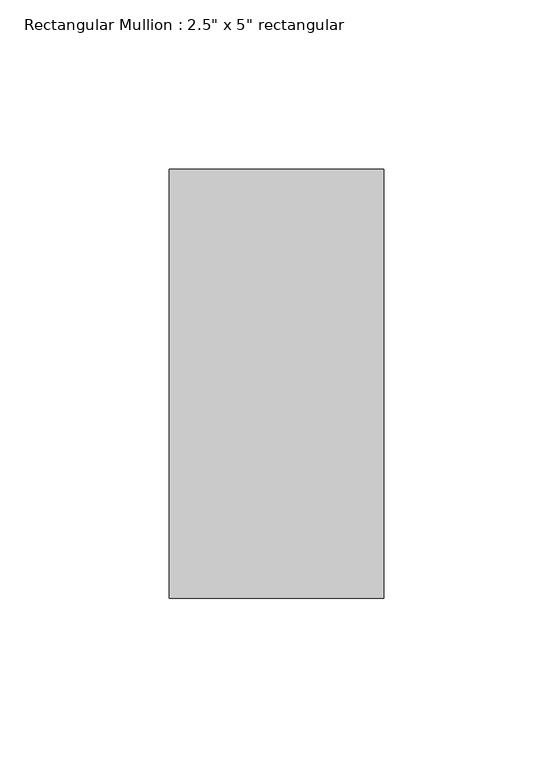
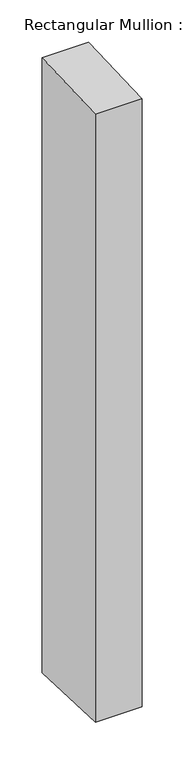
"""IFC4 building model written with IfcOpenShell, lengths in millimetres: member geometry."""

from ifc_helpers import new_model, si_unit, frame, origin, place, context, project, spatial, polyline, outline, extrude, source, transform, mapped, element, save


def member_b12940b7(model_context):
    return source(origin(), model_context, "Body", "SweptSolid", [
        extrude(outline(polyline([(-63.5, -2.5814971), (63.5, 2.5814971), (63.5, -887.2980727), (-63.5, -882.1350785), (-63.5, -2.5814971)])), frame((-63.5, 0.0, 0.0), z_axis=(1.0, 0.0, 0.0), x_axis=(0.0, 1.0, 0.0)), (0.0, 0.0, 1.0), 63.5),
    ])


if __name__ == "__main__":
    model = new_model("IFC4")
    model_context = context("Model", 3, world=origin())
    ifc_project = project(units=[si_unit("LENGTHUNIT", "METRE", prefix="MILLI")], contexts=[model_context])
    site = spatial("IfcSite", under=ifc_project)
    building = spatial("IfcBuilding", under=site)
    placement = place(None, origin())
    member_shape = member_b12940b7(model_context)
    element("IfcMember", 1, ObjectType="Rectangular Mullion : 2.5\" x 5\" rectangular", at=placement, inside=building, context=model_context, shape_type="MappedRepresentation", body=[
        mapped(member_shape, transform((0.0, 0.0, 0.0), x_axis=(1.0, 0.0, 0.0), y_axis=(0.0, 1.0, 0.0), z_axis=(0.0, 0.0, 1.0))),
    ])
    save(model, "model.ifc")

# Revit data of these elements
# Type "Rectangular Mullion : 2.5\" x 5\" rectangular"
#   built-in parameter 1007304 = 0.416667 (stored number, unit not read)
#   built-in parameter 1007301 = 0.104167 (stored number, unit not read)
#   built-in parameter 1007300 = 0.104167 (stored number, unit not read)
# Element 1 (IfcMember, "Rectangular Mullion : 2.5\" x 5\" rectangular")
#   Materials on its faces: "Aluminum"
# Materials
#   "Aluminum": class "Metal", colour RGB 247 247 247, transparency 0, Description = "Aluminum 6061", Cost = 0
